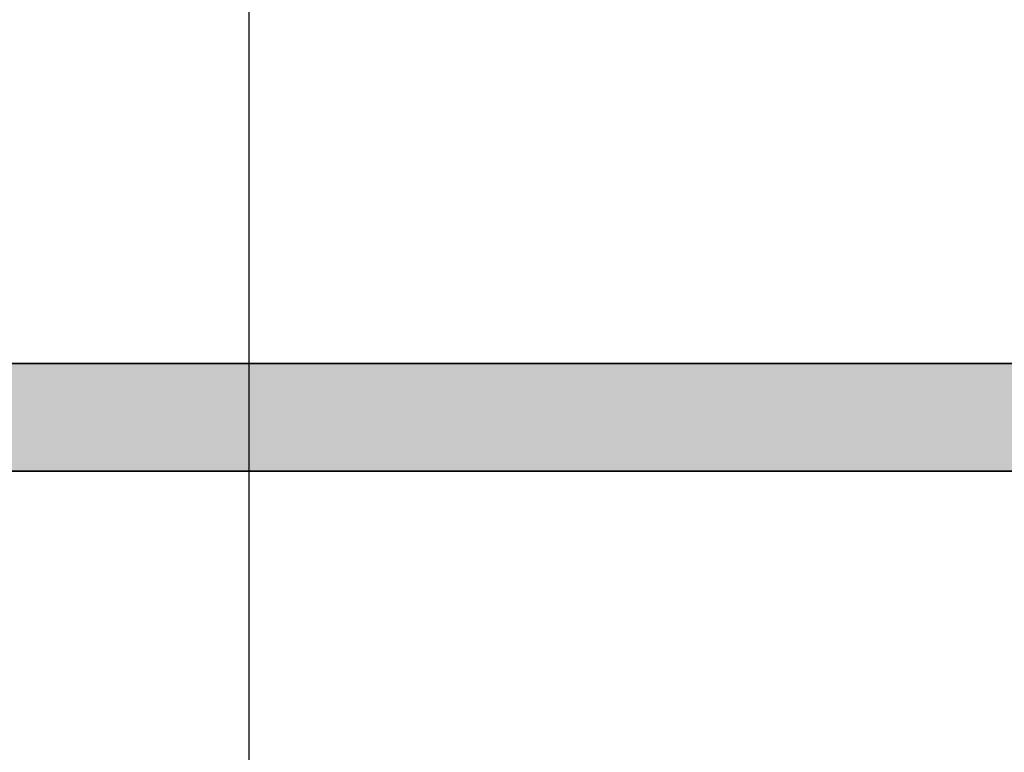
# Model space of a CAD drawing. Units: inches. Extents: x 2696 to 3240, y 1564 to 2310.
# Tile 74 of 76: x 3127 to 3168, y 2111 to 2142. Entities that reach past the tile are written whole.
import ezdxf

# ---------------------------------------------------------------- set-up
doc = ezdxf.new("R2010")
doc.units = ezdxf.units.IN
for name, color, linetype, lineweight in [('A-ANNO-DIMS', 3, 'Continuous', 18), ('A-WALL', 7, 'Continuous', 35), ('A-WALL-PATT', 9, 'Continuous', 13)]:
    doc.layers.add(name, color=color, linetype=linetype, lineweight=lineweight)
doc.styles.add('TIMES NEW', font='times.ttf')
doc.dimstyles.new('Siddhuu', dxfattribs={"dimtxt": 6, "dimasz": 2.5, "dimexe": 1.25, "dimexo": 0.625, "dimtad": 1, "dimdec": 1, "dimlunit": 4, "dimtxsty": 'TIMES NEW', "dimcen": 2.5, "dimclrd": 256, "dimclre": 1, "dimclrt": 7, "dimadec": 0, "dimazin": 0, "dimtfac": 1, "dimtdec": 1, "dimtmove": 0, "dimatfit": 3, "dimfxl": 1, "dimtolj": 1, "dimlwd": -1, "dimarcsym": 0})

# ---------------------------------------------------------------- blocks, each defined once
blk = doc.blocks.new('*D54')
at = {"layer": 'A-ANNO-DIMS', "color": 1, "lineweight": -2, "transparency": 16777216}
for p, q in [((3124.611, 1893.826), (3124.611, 2298.451)), ((3136.611, 1893.826), (3136.611, 2298.451))]:
    blk.add_line(p, q, dxfattribs=at)
at = {"layer": 'A-ANNO-DIMS', "transparency": 16777216}
for p, q in [((3127.111, 2297.201), (3134.111, 2297.201)), ((3136.611, 2297.201), (3155.757, 2297.201))]:
    blk.add_line(p, q, dxfattribs=at)
for points in [[(3127.111, 2297.618), (3127.111, 2296.784), (3124.611, 2297.201)], [(3134.111, 2297.618), (3134.111, 2296.784), (3136.611, 2297.201)]]:
    blk.add_solid(points, dxfattribs=at)
at = {"layer": 'Defpoints', "color": 0, "transparency": 16777216}
for p in [(3136.611, 2297.201), (3124.611, 1893.201), (3136.611, 1893.201)]:
    blk.add_point(p, dxfattribs=at)
at = {"layer": 'A-ANNO-DIMS', "color": 7, "transparency": 16777216, "insert": (3147.434, 2300.878), "char_height": 6, "attachment_point": 5, "style": 'TIMES NEW'}
blk.add_mtext('\\A1;1\'-0"', dxfattribs=at)

msp = doc.modelspace()

# ---------------------------------------------------------------- hatches: boundary and pattern name
at = {"layer": 'A-WALL-PATT', "transparency": 33554556}
h = msp.add_hatch(color=256, dxfattribs=at)
h.dxf.hatch_style = 1
h.paths.add_polyline_path([(2879.111, 2253.201), (2905.91, 2253.201), (2905.91, 2262.201), (2841.889, 2262.201), (2841.889, 2253.201), (2870.111, 2253.201), (2870.111, 2176.601), (2965.709, 2176.601), (2965.709, 2206.701), (2973.583, 2206.701), (2973.583, 2215.701), (2965.709, 2215.701), (2965.709, 2262.201), (2929.91, 2262.201), (2929.91, 2253.201), (2956.709, 2253.201), (2956.709, 2185.601), (2879.111, 2185.601)])
h.paths.add_polyline_path([(2782.834, 2262.201), (2745.611, 2262.201), (2745.611, 2228.729), (2754.611, 2228.729), (2754.611, 2253.201), (2782.834, 2253.201)])
h.paths.add_polyline_path([(2754.611, 2136.201), (2965.709, 2136.201), (2965.709, 2145.201), (2879.111, 2145.201), (2879.111, 2147.074), (2877.34, 2147.074), (2870.111, 2147.074), (2870.111, 2145.201), (2754.611, 2145.201), (2754.611, 2169.674), (2745.611, 2169.674), (2745.611, 2000.201), (2754.611, 2000.201), (2754.611, 2019.201), (2849.083, 2019.201), (2849.083, 2023.701), (2841.209, 2023.701), (2841.209, 2051.827), (2836.709, 2051.827), (2836.709, 2023.701), (2754.611, 2023.701), (2754.611, 2091.201), (2836.709, 2091.201), (2836.709, 2087.827), (2841.209, 2087.827), (2841.209, 2095.701), (2754.611, 2095.701)])
h.paths.add_polyline_path([(2965.709, 2136.201), (2956.709, 2136.201), (2956.709, 2023.701), (2885.083, 2023.701), (2885.083, 2019.201), (2956.709, 2019.201), (2956.709, 1950.575), (2965.709, 1950.575), (2965.709, 1980.201), (2973.583, 1980.201), (2973.583, 1989.201), (2965.709, 1989.201)])
h.paths.add_polyline_path([(2754.611, 1906.701), (2880.209, 1906.701), (2884.709, 1906.701), (2956.709, 1906.701), (2956.709, 1792.701), (2944.709, 1792.701), (2944.709, 1783.701), (2956.709, 1783.701), (2956.709, 1740.201), (2884.709, 1740.201), (2884.709, 1783.701), (2896.709, 1783.701), (2896.709, 1792.701), (2884.709, 1792.701), (2884.709, 1846.701), (2880.209, 1846.701), (2880.209, 1740.201), (2754.611, 1740.201), (2754.611, 1777.201), (2745.611, 1777.201), (2745.611, 1692.701), (2754.611, 1692.701), (2754.611, 1731.201), (2956.709, 1731.201), (2956.709, 1723.327), (2965.709, 1723.327), (2965.709, 1884.201), (2973.583, 1884.201), (2973.583, 1893.201), (2965.709, 1893.201), (2965.709, 1914.575), (2956.709, 1914.575), (2956.709, 1911.201), (2754.611, 1911.201), (2754.611, 1930.201), (2745.611, 1930.201), (2745.611, 1817.201), (2754.611, 1817.201), (2754.611, 1854.201), (2826.611, 1854.201), (2826.611, 1868.827), (2822.111, 1868.827), (2822.111, 1858.701), (2754.611, 1858.701)])
h.paths.add_polyline_path([(2965.709, 1656.201), (3008.237, 1656.201), (3008.237, 1665.201), (2965.709, 1665.201), (2965.709, 1693.327), (2956.709, 1693.327), (2956.709, 1686.201), (2934.583, 1686.201), (2934.583, 1681.701), (2956.709, 1681.701), (2956.709, 1614.201), (2896.709, 1614.201), (2896.709, 1681.701), (2904.583, 1681.701), (2904.583, 1686.201), (2892.209, 1686.201), (2892.209, 1614.201), (2858.41, 1614.201), (2858.41, 1605.201), (2965.709, 1605.201)])
h.paths.add_polyline_path([(2788.41, 1614.201), (2754.611, 1614.201), (2754.611, 1652.701), (2745.611, 1652.701), (2745.611, 1605.201), (2788.41, 1605.201)])
h.paths.add_polyline_path([(3199.611, 1633.048), (3190.611, 1633.048), (3190.611, 1614.201), (3082.611, 1614.201), (3082.611, 1665.201), (3070.237, 1665.201), (3070.237, 1656.201), (3078.111, 1656.201), (3078.111, 1605.201), (3199.611, 1605.201)])
h.paths.add_polyline_path([(3199.611, 1702.048), (3190.611, 1702.048), (3190.611, 1699.701), (3106.611, 1699.701), (3106.611, 1747.701), (3190.611, 1747.701), (3190.611, 1752.201), (3082.611, 1752.201), (3082.611, 1760.075), (3078.111, 1760.075), (3078.111, 1747.701), (3102.111, 1747.701), (3102.111, 1699.701), (3078.111, 1699.701), (3078.111, 1695.201), (3190.611, 1695.201), (3190.611, 1676.355), (3199.611, 1676.355)])
h.paths.add_polyline_path([(3199.611, 1783.201), (3190.611, 1783.201), (3190.611, 1745.355), (3199.611, 1745.355)])
h.paths.add_polyline_path([(3082.611, 1884.201), (3190.611, 1884.201), (3190.611, 1853.201), (3199.611, 1853.201), (3199.611, 1901.701), (3190.611, 1901.701), (3190.611, 1893.201), (3005.583, 1893.201), (3005.583, 1891.281), (3005.583, 1884.201), (3078.111, 1884.201), (3078.111, 1792.075), (3082.611, 1792.075)])
h.paths.add_polyline_path([(3199.611, 1994.701), (3190.611, 1994.701), (3190.611, 1989.201), (3073.709, 1989.201), (3073.709, 2034.201), (3069.209, 2034.201), (3069.209, 1989.201), (3005.583, 1989.201), (3005.583, 1980.201), (3190.611, 1980.201), (3190.611, 1971.701), (3199.611, 1971.701)])
h.paths.add_polyline_path([(3199.611, 2155.201), (3190.611, 2155.201), (3190.611, 2064.701), (3199.611, 2064.701)])
h.paths.add_polyline_path([(3190.611, 2074.701), (3106.611, 2074.701), (3106.611, 2122.701), (3190.611, 2122.701), (3190.611, 2127.201), (3082.709, 2127.201), (3082.709, 2135.075), (3073.709, 2135.075), (3073.709, 2122.701), (3102.111, 2122.701), (3102.111, 2074.701), (3069.209, 2074.701), (3069.209, 2070.201), (3190.611, 2070.201)])
h.paths.add_polyline_path([(3082.709, 2253.201), (3190.611, 2253.201), (3190.611, 2225.201), (3199.611, 2225.201), (3199.611, 2262.201), (3073.709, 2262.201), (3073.709, 2215.701), (3035.583, 2215.701), (3035.583, 2206.701), (3073.709, 2206.701), (3073.709, 2171.075), (3082.709, 2171.075)])

# ---------------------------------------------------------------- linework, layer by layer
at = {"layer": 'A-WALL'}
for p, q in [((3082.709, 2127.201), (3190.611, 2127.201)), ((3106.611, 2122.701), (3190.611, 2122.701))]:
    msp.add_line(p, q, dxfattribs=at)

# ---------------------------------------------------------------- dimensions: what is measured, and where the dimension line sits
at = {"layer": 'A-ANNO-DIMS'}
dim = msp.add_linear_dim(base=(3136.611, 2297.201), p1=(3124.611, 1893.201), p2=(3136.611, 1893.201), dimstyle='Siddhuu', override={"dimdec": 1, "dimlfac": 1, "dimrnd": 0, "dimzin": 1, "dimdsep": 46, "dimlunit": 4, "dimfrac": 2}, dxfattribs=at)
dim.commit()
dim.dimension.update_dxf_attribs({"geometry": '*D54', "text_midpoint": (3147.434, 2300.878)})

doc.saveas('drawing.dxf')
